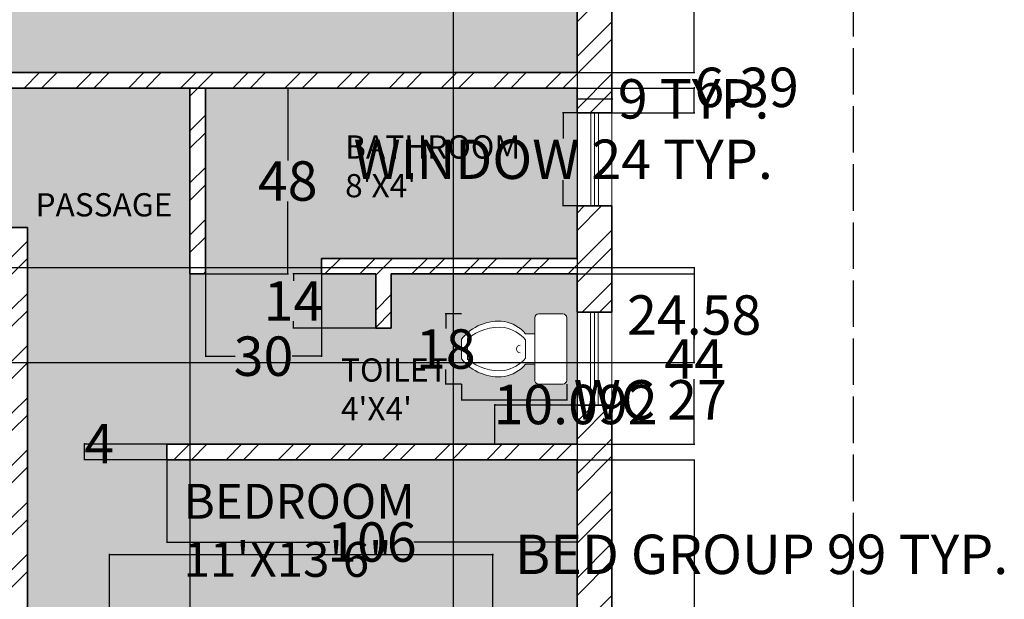
# Model space of a CAD drawing. Units: inches. Extents: x 1410 to 1959, y 5441 to 5968.
# Tile 4 of 5: x 1705 to 1959, y 5615 to 5765. Entities that reach past the tile are written whole.
import ezdxf

# ---------------------------------------------------------------- set-up
doc = ezdxf.new("R2010")
doc.units = ezdxf.units.IN
doc.linetypes.add('ACAD_ISO02W100', pattern=[15, 12, -3])
doc.layers.get('Defpoints').update_dxf_attribs({"linetype": 'ACAD_ISO02W100'})
for name, color, linetype, lineweight in [('A-ANNO-DIMS', 2, 'Continuous', 18), ('A-AREA-IDEN', 7, 'Continuous', 18), ('A-FLOR-FIXT', 9, 'Continuous', 18), ('A-WALL', 7, 'Continuous', 35), ('A-WALL-PATT', 8, 'Continuous', 13), ('WINDOW', 160, 'Continuous', 13)]:
    doc.layers.add(name, color=color, linetype=linetype, lineweight=lineweight)
doc.layers.add('A-FLOR-PATT', color=9, linetype='Continuous', lineweight=9, true_color=0xafd9aa)
doc.styles.get("Standard").update_dxf_attribs({"font": 'arial.ttf'})
doc.dimstyles.get("Standard").update_dxf_attribs({"dimtxt": 10.18, "dimasz": 0.18, "dimexe": 0.18, "dimexo": 0.0625, "dimgap": 0.09, "dimtad": 0, "dimtih": 1, "dimtoh": 1, "dimdec": 0, "dimzin": 0, "dimdsep": 46, "dimlunit": 3, "dimtxsty": 'Standard', "dimcen": 0.09, "dimadec": 0, "dimazin": 0, "dimtfac": 1, "dimtdec": 0, "dimtofl": 0, "dimtmove": 0, "dimatfit": 3, "dimfxl": 1, "dimtolj": 1, "dimtzin": 0, "dimarcsym": 0})

# ---------------------------------------------------------------- blocks, each defined once
blk = doc.blocks.new('A$C2AC94788')
for p, q in [((0, 0.505), (0, 0.665)), ((0.025, 0.69), (0.435, 0.69)), ((0.46, 0.665), (0.46, 0.505)), ((0.435, 0.48), (0.025, 0.48)), ((0.13, 0.48), (0.13, 0.42)), ((0.33, 0.42), (0.33, 0.48)), ((0.17, 0.42), (0.29, 0.42)), ((0.1641, 0.0392), (0.2959, 0.0392)), ((0.2291, 0.0392), (0.23, 0.0392)), ((0.2309, 0.0392), (0.23, 0.0392)), ((0.165, 0), (0.295, 0))]:
    blk.add_line(p, q)
for centre, radius, start, end in [((0.025, 0.665), 0.025, 90, 180), ((0.435, 0.665), 0.025, 0, 90), ((0.025, 0.505), 0.025, 180, 270), ((0.435, 0.505), 0.025, 270, 0), ((0.2874, 0.2356), 0.2425, 130.48854, 169.44501), ((0.3274, 0.2356), 0.2425, 130.48854, 169.44501), ((0.1326, 0.2356), 0.2425, 10.55499, 49.51146), ((0.1726, 0.2356), 0.2425, 10.55499, 49.51146), ((0.23, 0.385), 0.025, 180, 0), ((0.3601, 0.2448), 0.313, 173.53688, 231.44828), ((0.4001, 0.2448), 0.313, 173.53688, 221.06038), ((0.0999, 0.2448), 0.313, 308.55172, 6.46312), ((0.0599, 0.2448), 0.313, 318.93962, 6.46312)]:
    blk.add_arc(centre, radius, start, end)
blk = doc.blocks.new('WIN-24IN')
for p, q in [((3.5, 24), (3.5, 0)), ((4.5, 24), (4.5, 0)), ((5.5, 24), (5.5, 0))]:
    blk.add_line(p, q)
blk.add_lwpolyline([(0, 0), (9, 0), (9, 24), (0, 24)], close=True)
blk = doc.blocks.new('*D12')
at = {"layer": 'A-ANNO-DIMS', "color": 0, "lineweight": -2, "transparency": 16777216}
for p, q in [((1849.06, 5740.98), (1845.34, 5740.98)), ((1845.52, 5740.8), (1845.52, 5734.33)), ((1845.52, 5717.16), (1845.52, 5723.62)), ((1849.06, 5716.98), (1845.34, 5716.98))]:
    blk.add_line(p, q, dxfattribs=at)
at = {"layer": 'A-ANNO-DIMS', "color": 0, "transparency": 16777216}
for points in [[(1845.49, 5740.8), (1845.55, 5740.8), (1845.52, 5740.98)], [(1845.49, 5717.16), (1845.55, 5717.16), (1845.52, 5716.98)]]:
    blk.add_solid(points, dxfattribs=at)
at = {"layer": 'Defpoints', "color": 0, "transparency": 16777216}
for p in [(1845.52, 5740.98), (1849.12, 5740.98), (1849.12, 5716.98)]:
    blk.add_point(p, dxfattribs=at)
at = {"layer": 'A-ANNO-DIMS', "color": 0, "transparency": 16777216, "insert": (1845.52, 5728.98), "char_height": 10.18, "attachment_point": 5}
blk.add_mtext('\\A1;WINDOW 24 TYP.', dxfattribs=at)
blk = doc.blocks.new('*D13')
at = {"layer": 'A-ANNO-DIMS', "color": 0, "lineweight": -2, "transparency": 16777216}
for p, q in [((1849.12, 5741.04), (1849.12, 5744.76)), ((1849.3, 5744.58), (1857.94, 5744.58)), ((1858.12, 5741.04), (1858.12, 5744.76)), ((1858.12, 5744.58), (1858.3, 5744.58))]:
    blk.add_line(p, q, dxfattribs=at)
at = {"layer": 'A-ANNO-DIMS', "color": 0, "transparency": 16777216}
for points in [[(1849.3, 5744.61), (1849.3, 5744.55), (1849.12, 5744.58)], [(1857.94, 5744.61), (1857.94, 5744.55), (1858.12, 5744.58)]]:
    blk.add_solid(points, dxfattribs=at)
at = {"layer": 'Defpoints', "color": 0, "transparency": 16777216}
for p in [(1858.12, 5744.58), (1849.12, 5740.98), (1858.12, 5740.98)]:
    blk.add_point(p, dxfattribs=at)
at = {"layer": 'A-ANNO-DIMS', "color": 0, "transparency": 16777216, "insert": (1879.21, 5744.58), "char_height": 10.18, "attachment_point": 5}
blk.add_mtext('\\A1;9 TYP.', dxfattribs=at)
blk = doc.blocks.new('*D14')
at = {"layer": 'A-ANNO-DIMS', "color": 0, "lineweight": -2, "transparency": 16777216}
for p, q in [((1728.31, 5612.14), (1728.31, 5627.11)), ((1728.49, 5626.93), (1827.13, 5626.93)), ((1827.31, 5612.14), (1827.31, 5627.11)), ((1827.31, 5626.93), (1827.49, 5626.93))]:
    blk.add_line(p, q, dxfattribs=at)
at = {"layer": 'A-ANNO-DIMS', "color": 0, "transparency": 16777216}
for points in [[(1728.49, 5626.96), (1728.49, 5626.9), (1728.31, 5626.93)], [(1827.13, 5626.96), (1827.13, 5626.9), (1827.31, 5626.93)]]:
    blk.add_solid(points, dxfattribs=at)
at = {"layer": 'Defpoints', "color": 0, "transparency": 16777216}
for p in [(1827.31, 5626.93), (1728.31, 5612.08), (1827.31, 5612.08)]:
    blk.add_point(p, dxfattribs=at)
at = {"layer": 'A-ANNO-DIMS', "color": 0, "transparency": 16777216, "insert": (1896.77, 5626.93), "char_height": 10.18, "attachment_point": 5}
blk.add_mtext('\\A1;BED GROUP 99 TYP.', dxfattribs=at)
blk = doc.blocks.new('*D22')
at = {"layer": 'A-ANNO-DIMS', "color": 0, "lineweight": -2, "transparency": 16777216}
for p, q in [((1819.26, 5670.85), (1819.26, 5666.66)), ((1846.43, 5670.85), (1846.43, 5666.66)), ((1819.44, 5666.84), (1846.25, 5666.84)), ((1846.43, 5666.84), (1846.61, 5666.84))]:
    blk.add_line(p, q, dxfattribs=at)
at = {"layer": 'A-ANNO-DIMS', "color": 0, "transparency": 16777216}
for points in [[(1819.44, 5666.87), (1819.44, 5666.81), (1819.26, 5666.84)], [(1846.25, 5666.87), (1846.25, 5666.81), (1846.43, 5666.84)]]:
    blk.add_solid(points, dxfattribs=at)
at = {"layer": 'Defpoints', "color": 0, "transparency": 16777216}
for p in [(1819.26, 5670.92), (1846.43, 5670.92), (1846.43, 5666.84)]:
    blk.add_point(p, dxfattribs=at)
at = {"layer": 'A-ANNO-DIMS', "color": 0, "transparency": 16777216, "insert": (1868.02, 5666.84), "char_height": 10.18, "attachment_point": 5}
blk.add_mtext('\\A1;WC 27', dxfattribs=at)
blk = doc.blocks.new('*D23')
at = {"layer": 'A-ANNO-DIMS', "color": 0, "lineweight": -2, "transparency": 16777216}
for p, q in [((1819.2, 5689.03), (1815.01, 5689.03)), ((1815.19, 5688.85), (1815.19, 5685.26)), ((1815.19, 5671.1), (1815.19, 5674.68)), ((1819.2, 5670.92), (1815.01, 5670.92))]:
    blk.add_line(p, q, dxfattribs=at)
at = {"layer": 'A-ANNO-DIMS', "color": 0, "transparency": 16777216}
for points in [[(1815.16, 5688.85), (1815.22, 5688.85), (1815.19, 5689.03)], [(1815.16, 5671.1), (1815.22, 5671.1), (1815.19, 5670.92)]]:
    blk.add_solid(points, dxfattribs=at)
at = {"layer": 'Defpoints', "color": 0, "transparency": 16777216}
for p in [(1819.26, 5689.03), (1815.19, 5670.92), (1819.26, 5670.92)]:
    blk.add_point(p, dxfattribs=at)
at = {"layer": 'A-ANNO-DIMS', "color": 0, "transparency": 16777216, "insert": (1815.19, 5679.97), "char_height": 10.18, "attachment_point": 5}
blk.add_mtext('\\A1;18', dxfattribs=at)
blk = doc.blocks.new('*D28')
at = {"layer": 'A-ANNO-DIMS', "color": 0, "lineweight": -2, "transparency": 16777216}
for p, q in [((1817.1, 5913.3), (1817.1, 5478.87)), ((1849.09, 5913.3), (1849.09, 5478.87)), ((1817.28, 5479.05), (1848.91, 5479.05)), ((1849.09, 5479.05), (1849.27, 5479.05))]:
    blk.add_line(p, q, dxfattribs=at)
at = {"layer": 'A-ANNO-DIMS', "color": 0, "transparency": 16777216}
for points in [[(1817.28, 5479.08), (1817.28, 5479.02), (1817.1, 5479.05)], [(1848.91, 5479.08), (1848.91, 5479.02), (1849.09, 5479.05)]]:
    blk.add_solid(points, dxfattribs=at)
at = {"layer": 'Defpoints', "color": 0, "transparency": 16777216}
for p in [(1817.1, 5913.37), (1849.09, 5913.37), (1849.09, 5479.05)]:
    blk.add_point(p, dxfattribs=at)
at = {"layer": 'A-ANNO-DIMS', "color": 0, "transparency": 16777216, "insert": (1866.55, 5479.05), "char_height": 10.18, "attachment_point": 5}
blk.add_mtext('\\A1;31.99', dxfattribs=at)
blk = doc.blocks.new('*D32')
at = {"layer": 'A-ANNO-DIMS', "color": 0, "lineweight": -2, "transparency": 16777216}
for p, q in [((1849.03, 5665.46), (1827.66, 5665.46)), ((1827.84, 5665.46), (1827.84, 5665.64)), ((1827.84, 5665.64), (1828.02, 5665.64)), ((1827.84, 5655.55), (1827.84, 5665.28)), ((1849.03, 5655.37), (1827.66, 5655.37))]:
    blk.add_line(p, q, dxfattribs=at)
at = {"layer": 'A-ANNO-DIMS', "color": 0, "transparency": 16777216}
for points in [[(1827.81, 5665.28), (1827.87, 5665.28), (1827.84, 5665.46)], [(1827.81, 5655.55), (1827.87, 5655.55), (1827.84, 5655.37)]]:
    blk.add_solid(points, dxfattribs=at)
at = {"layer": 'Defpoints', "color": 0, "transparency": 16777216}
for p in [(1827.84, 5665.46), (1849.09, 5665.46), (1849.09, 5655.37)]:
    blk.add_point(p, dxfattribs=at)
at = {"layer": 'A-ANNO-DIMS', "color": 0, "transparency": 16777216, "insert": (1848.71, 5665.64), "char_height": 10.18, "attachment_point": 5}
blk.add_mtext('\\A1;10.092', dxfattribs=at)
blk = doc.blocks.new('*D33')
at = {"layer": 'A-ANNO-DIMS', "color": 0, "lineweight": -2, "transparency": 16777216}
for p, q in [((1849.16, 5747.37), (1879.55, 5747.37)), ((1879.37, 5747.37), (1879.37, 5747.55)), ((1879.37, 5747.55), (1879.55, 5747.55)), ((1879.37, 5741.16), (1879.37, 5747.19)), ((1849.19, 5740.98), (1879.55, 5740.98))]:
    blk.add_line(p, q, dxfattribs=at)
at = {"layer": 'A-ANNO-DIMS', "color": 0, "transparency": 16777216}
for points in [[(1879.34, 5747.19), (1879.4, 5747.19), (1879.37, 5747.37)], [(1879.34, 5741.16), (1879.4, 5741.16), (1879.37, 5740.98)]]:
    blk.add_solid(points, dxfattribs=at)
at = {"layer": 'Defpoints', "color": 0, "transparency": 16777216}
for p in [(1849.09, 5747.37), (1879.37, 5747.37), (1849.12, 5740.98)]:
    blk.add_point(p, dxfattribs=at)
at = {"layer": 'A-ANNO-DIMS', "color": 0, "transparency": 16777216, "insert": (1892.9, 5747.55), "char_height": 10.18, "attachment_point": 5}
blk.add_mtext('\\A1;6.39', dxfattribs=at)
blk = doc.blocks.new('*D41')
at = {"layer": 'A-ANNO-DIMS', "color": 0, "lineweight": -2, "transparency": 16777216}
for p, q in [((1849.16, 5651.37), (1879.55, 5651.37)), ((1879.37, 5651.19), (1879.37, 5598.65)), ((1879.37, 5535.55), (1879.37, 5588.08)), ((1849.16, 5535.37), (1879.55, 5535.37))]:
    blk.add_line(p, q, dxfattribs=at)
at = {"layer": 'A-ANNO-DIMS', "color": 0, "transparency": 16777216}
for points in [[(1879.34, 5651.19), (1879.4, 5651.19), (1879.37, 5651.37)], [(1879.34, 5535.55), (1879.4, 5535.55), (1879.37, 5535.37)]]:
    blk.add_solid(points, dxfattribs=at)
at = {"layer": 'Defpoints', "color": 0, "transparency": 16777216}
for p in [(1849.09, 5651.37), (1879.37, 5651.37), (1849.09, 5535.37)]:
    blk.add_point(p, dxfattribs=at)
at = {"layer": 'A-ANNO-DIMS', "color": 0, "transparency": 16777216, "insert": (1879.37, 5593.37), "char_height": 10.18, "attachment_point": 5}
blk.add_mtext('\\A1;116', dxfattribs=at)
blk = doc.blocks.new('*D43')
at = {"layer": 'A-ANNO-DIMS', "color": 0, "lineweight": -2, "transparency": 16777216}
for p, q in [((1849.16, 5913.37), (1879.55, 5913.37)), ((1879.37, 5913.19), (1879.37, 5837.65)), ((1879.37, 5751.55), (1879.37, 5827.08)), ((1849.16, 5751.37), (1879.55, 5751.37))]:
    blk.add_line(p, q, dxfattribs=at)
at = {"layer": 'A-ANNO-DIMS', "color": 0, "transparency": 16777216}
for points in [[(1879.34, 5913.19), (1879.4, 5913.19), (1879.37, 5913.37)], [(1879.34, 5751.55), (1879.4, 5751.55), (1879.37, 5751.37)]]:
    blk.add_solid(points, dxfattribs=at)
at = {"layer": 'Defpoints', "color": 0, "transparency": 16777216}
for p in [(1849.09, 5913.37), (1879.37, 5913.37), (1849.09, 5751.37)]:
    blk.add_point(p, dxfattribs=at)
at = {"layer": 'A-ANNO-DIMS', "color": 0, "transparency": 16777216, "insert": (1879.37, 5832.37), "char_height": 10.18, "attachment_point": 5}
blk.add_mtext('\\A1;162', dxfattribs=at)
blk = doc.blocks.new('*D44')
at = {"layer": 'A-ANNO-DIMS', "color": 0, "lineweight": -2, "transparency": 16777216}
for p, q in [((1753.09, 5699.3), (1753.09, 5677.94)), ((1783.09, 5699.3), (1783.09, 5677.94)), ((1753.27, 5678.12), (1760.73, 5678.12)), ((1782.91, 5678.12), (1775.45, 5678.12))]:
    blk.add_line(p, q, dxfattribs=at)
at = {"layer": 'A-ANNO-DIMS', "color": 0, "transparency": 16777216}
for points in [[(1753.27, 5678.15), (1753.27, 5678.09), (1753.09, 5678.12)], [(1782.91, 5678.15), (1782.91, 5678.09), (1783.09, 5678.12)]]:
    blk.add_solid(points, dxfattribs=at)
at = {"layer": 'Defpoints', "color": 0, "transparency": 16777216}
for p in [(1753.09, 5699.37), (1783.09, 5699.37), (1753.09, 5678.12)]:
    blk.add_point(p, dxfattribs=at)
at = {"layer": 'A-ANNO-DIMS', "color": 0, "transparency": 16777216, "insert": (1768.09, 5678.12), "char_height": 10.18, "attachment_point": 5}
blk.add_mtext('\\A1;30', dxfattribs=at)
blk = doc.blocks.new('*D45')
at = {"layer": 'A-ANNO-DIMS', "color": 0, "lineweight": -2, "transparency": 16777216}
for p, q in [((1797.03, 5699.37), (1775.66, 5699.37)), ((1775.84, 5699.19), (1775.84, 5697.57)), ((1775.84, 5685.55), (1775.84, 5687.17)), ((1797.03, 5685.37), (1775.66, 5685.37))]:
    blk.add_line(p, q, dxfattribs=at)
at = {"layer": 'A-ANNO-DIMS', "color": 0, "transparency": 16777216}
for points in [[(1775.81, 5699.19), (1775.87, 5699.19), (1775.84, 5699.37)], [(1775.81, 5685.55), (1775.87, 5685.55), (1775.84, 5685.37)]]:
    blk.add_solid(points, dxfattribs=at)
at = {"layer": 'Defpoints', "color": 0, "transparency": 16777216}
for p in [(1775.84, 5699.37), (1797.09, 5699.37), (1797.09, 5685.37)]:
    blk.add_point(p, dxfattribs=at)
at = {"layer": 'A-ANNO-DIMS', "color": 0, "transparency": 16777216, "insert": (1775.84, 5692.37), "char_height": 10.18, "attachment_point": 5}
blk.add_mtext('\\A1;14', dxfattribs=at)
blk = doc.blocks.new('*D46')
at = {"layer": 'A-ANNO-DIMS', "color": 0, "lineweight": -2, "transparency": 16777216}
for p, q in [((1707.09, 5711.3), (1707.09, 5478.87)), ((1749.09, 5699.3), (1749.09, 5478.87)), ((1707.27, 5479.05), (1720.56, 5479.05)), ((1748.91, 5479.05), (1735.63, 5479.05))]:
    blk.add_line(p, q, dxfattribs=at)
at = {"layer": 'A-ANNO-DIMS', "color": 0, "transparency": 16777216}
for points in [[(1707.27, 5479.08), (1707.27, 5479.02), (1707.09, 5479.05)], [(1748.91, 5479.08), (1748.91, 5479.02), (1749.09, 5479.05)]]:
    blk.add_solid(points, dxfattribs=at)
at = {"layer": 'Defpoints', "color": 0, "transparency": 16777216}
for p in [(1707.09, 5711.37), (1749.09, 5699.37), (1749.09, 5479.05)]:
    blk.add_point(p, dxfattribs=at)
at = {"layer": 'A-ANNO-DIMS', "color": 0, "transparency": 16777216, "insert": (1728.09, 5479.05), "char_height": 10.18, "attachment_point": 5}
blk.add_mtext('\\A1;42', dxfattribs=at)
blk = doc.blocks.new('*D47')
at = {"layer": 'A-ANNO-DIMS', "color": 0, "lineweight": -2, "transparency": 16777216}
for p, q in [((1707.03, 5747.37), (1685.66, 5747.37)), ((1685.84, 5747.19), (1685.84, 5734.66)), ((1685.84, 5711.55), (1685.84, 5724.07)), ((1707.03, 5711.37), (1685.66, 5711.37))]:
    blk.add_line(p, q, dxfattribs=at)
at = {"layer": 'A-ANNO-DIMS', "color": 0, "transparency": 16777216}
for points in [[(1685.81, 5747.19), (1685.87, 5747.19), (1685.84, 5747.37)], [(1685.81, 5711.55), (1685.87, 5711.55), (1685.84, 5711.37)]]:
    blk.add_solid(points, dxfattribs=at)
at = {"layer": 'Defpoints', "color": 0, "transparency": 16777216}
for p in [(1685.84, 5747.37), (1707.09, 5747.37), (1707.09, 5711.37)]:
    blk.add_point(p, dxfattribs=at)
at = {"layer": 'A-ANNO-DIMS', "color": 0, "transparency": 16777216, "insert": (1685.84, 5729.37), "char_height": 10.18, "attachment_point": 5}
blk.add_mtext('\\A1;36', dxfattribs=at)
blk = doc.blocks.new('*D48')
at = {"layer": 'A-ANNO-DIMS', "color": 0, "lineweight": -2, "transparency": 16777216}
for p, q in [((1743.09, 5651.3), (1743.09, 5629.94)), ((1849.09, 5651.3), (1849.09, 5629.94)), ((1743.27, 5630.12), (1785.24, 5630.12)), ((1848.91, 5630.12), (1806.95, 5630.12))]:
    blk.add_line(p, q, dxfattribs=at)
at = {"layer": 'A-ANNO-DIMS', "color": 0, "transparency": 16777216}
for points in [[(1743.27, 5630.15), (1743.27, 5630.09), (1743.09, 5630.12)], [(1848.91, 5630.15), (1848.91, 5630.09), (1849.09, 5630.12)]]:
    blk.add_solid(points, dxfattribs=at)
at = {"layer": 'Defpoints', "color": 0, "transparency": 16777216}
for p in [(1743.09, 5651.37), (1849.09, 5651.37), (1743.09, 5630.12)]:
    blk.add_point(p, dxfattribs=at)
at = {"layer": 'A-ANNO-DIMS', "color": 0, "transparency": 16777216, "insert": (1796.09, 5630.12), "char_height": 10.18, "attachment_point": 5}
blk.add_mtext('\\A1;106', dxfattribs=at)
blk = doc.blocks.new('*D56')
at = {"layer": 'A-ANNO-DIMS', "color": 0, "lineweight": -2, "transparency": 16777216}
for p, q in [((1743.03, 5655.37), (1721.66, 5655.37)), ((1721.84, 5655.37), (1721.84, 5655.55)), ((1721.84, 5655.55), (1722.02, 5655.55)), ((1721.84, 5651.55), (1721.84, 5655.19)), ((1743.03, 5651.37), (1721.66, 5651.37))]:
    blk.add_line(p, q, dxfattribs=at)
at = {"layer": 'A-ANNO-DIMS', "color": 0, "transparency": 16777216}
for points in [[(1721.81, 5655.19), (1721.87, 5655.19), (1721.84, 5655.37)], [(1721.81, 5651.55), (1721.87, 5651.55), (1721.84, 5651.37)]]:
    blk.add_solid(points, dxfattribs=at)
at = {"layer": 'Defpoints', "color": 0, "transparency": 16777216}
for p in [(1721.84, 5655.37), (1743.09, 5655.37), (1743.09, 5651.37)]:
    blk.add_point(p, dxfattribs=at)
at = {"layer": 'A-ANNO-DIMS', "color": 0, "transparency": 16777216, "insert": (1725.63, 5655.55), "char_height": 10.18, "attachment_point": 5}
blk.add_mtext('\\A1;4', dxfattribs=at)
blk = doc.blocks.new('*D57')
at = {"layer": 'A-ANNO-DIMS', "color": 0, "lineweight": -2, "transparency": 16777216}
for p, q in [((1753.16, 5747.37), (1774.52, 5747.37)), ((1774.34, 5747.19), (1774.34, 5728.65)), ((1774.34, 5699.55), (1774.34, 5718.08)), ((1753.16, 5699.37), (1774.52, 5699.37))]:
    blk.add_line(p, q, dxfattribs=at)
at = {"layer": 'A-ANNO-DIMS', "color": 0, "transparency": 16777216}
for points in [[(1774.31, 5747.19), (1774.37, 5747.19), (1774.34, 5747.37)], [(1774.31, 5699.55), (1774.37, 5699.55), (1774.34, 5699.37)]]:
    blk.add_solid(points, dxfattribs=at)
at = {"layer": 'Defpoints', "color": 0, "transparency": 16777216}
for p in [(1753.09, 5747.37), (1753.09, 5699.37), (1774.34, 5699.37)]:
    blk.add_point(p, dxfattribs=at)
at = {"layer": 'A-ANNO-DIMS', "color": 0, "transparency": 16777216, "insert": (1774.34, 5723.37), "char_height": 10.18, "attachment_point": 5}
blk.add_mtext('\\A1;48', dxfattribs=at)
blk = doc.blocks.new('*D58')
at = {"layer": 'A-ANNO-DIMS', "color": 0, "lineweight": -2, "transparency": 16777216}
for p, q in [((1849.156726, 5699.36591), (1879.553029, 5699.36591)), ((1879.373029, 5699.18591), (1879.373029, 5682.54591)), ((1879.373029, 5655.54591), (1879.373029, 5672.18591)), ((1849.156726, 5655.36591), (1879.553029, 5655.36591))]:
    blk.add_line(p, q, dxfattribs=at)
at = {"layer": 'A-ANNO-DIMS', "color": 0, "transparency": 16777216}
for points in [[(1879.343029, 5699.18591), (1879.403029, 5699.18591), (1879.373029, 5699.36591)], [(1879.343029, 5655.54591), (1879.403029, 5655.54591), (1879.373029, 5655.36591)]]:
    blk.add_solid(points, dxfattribs=at)
at = {"layer": 'Defpoints', "color": 0, "transparency": 16777216}
for p in [(1849.094226, 5699.36591), (1849.094226, 5655.36591), (1879.373029, 5655.36591)]:
    blk.add_point(p, dxfattribs=at)
at = {"layer": 'A-ANNO-DIMS', "color": 0, "transparency": 16777216, "insert": (1879.373029, 5677.36591), "char_height": 10.18, "attachment_point": 5}
blk.add_mtext('\\A1;44', dxfattribs=at)
blk = doc.blocks.new('*D59')
at = {"layer": 'A-ANNO-DIMS', "color": 0, "lineweight": -2, "transparency": 16777216}
for p, q in [((1559.15, 5701.04), (1879.55, 5701.04)), ((1879.37, 5700.86), (1879.37, 5694.04)), ((1879.37, 5676.64), (1879.37, 5683.46)), ((1559.15, 5676.46), (1879.55, 5676.46))]:
    blk.add_line(p, q, dxfattribs=at)
at = {"layer": 'A-ANNO-DIMS', "color": 0, "transparency": 16777216}
for points in [[(1879.34, 5700.86), (1879.4, 5700.86), (1879.37, 5701.04)], [(1879.34, 5676.64), (1879.4, 5676.64), (1879.37, 5676.46)]]:
    blk.add_solid(points, dxfattribs=at)
at = {"layer": 'Defpoints', "color": 0, "transparency": 16777216}
for p in [(1559.09, 5701.04), (1559.09, 5676.46), (1879.37, 5676.46)]:
    blk.add_point(p, dxfattribs=at)
at = {"layer": 'A-ANNO-DIMS', "color": 0, "transparency": 16777216, "insert": (1879.37, 5688.75), "char_height": 10.18, "attachment_point": 5}
blk.add_mtext('\\A1;24.58', dxfattribs=at)

msp = doc.modelspace()

# ---------------------------------------------------------------- hatches: boundary and pattern name
at = {"layer": 'A-FLOR-PATT', "transparency": 33554534}
h = msp.add_hatch(color=256, dxfattribs=at)
h.dxf.hatch_style = 1
h.paths.add_polyline_path([(1849.0942, 5913.3659), (1817.1029, 5913.3659), (1769.1029, 5913.3659), (1769.1029, 5913.3659), (1707.0942, 5913.3659), (1707.0942, 5787.3659), (1703.0942, 5787.3659), (1703.0942, 5799.3659), (1631.0942, 5799.3659), (1631.0942, 5787.3659), (1627.0942, 5787.3659), (1627.0942, 5889.3659), (1519.0989, 5889.3659), (1519.0989, 5816.4745), (1495.0981, 5816.4745), (1495.0981, 5809.856), (1495.0942, 5751.3659), (1631.0942, 5751.3659), (1631.0942, 5747.3659), (1495.0942, 5747.3659), (1495.0942, 5702.5811), (1495.0984, 5654.5768), (1495.0942, 5603.3659), (1667.0942, 5603.3659), (1667.0942, 5594.3659), (1650.778, 5594.3659), (1650.778, 5558.3659), (1703.0942, 5558.3659), (1703.0942, 5594.3659), (1703.0942, 5711.3659), (1707.0942, 5711.3659), (1707.0942, 5535.3659), (1754.5413, 5535.3659), (1802.541, 5535.3658), (1802.5413, 5535.3658), (1802.5413, 5535.3659), (1849.0942, 5535.3659), (1849.0942, 5651.3659), (1743.0942, 5651.3659), (1743.0942, 5655.3659), (1849.0942, 5655.3659), (1849.0942, 5665.4579), (1849.0942, 5689.4579), (1849.0942, 5699.3659), (1801.0942, 5699.3659), (1801.0942, 5685.3659), (1797.0942, 5685.3659), (1797.0942, 5699.3659), (1783.0942, 5699.3659), (1783.0942, 5703.3659), (1849.0942, 5703.3659), (1849.0942, 5716.9764), (1849.123, 5716.9764), (1849.123, 5740.9654), (1849.0942, 5740.9654), (1849.0942, 5747.3659), (1753.0942, 5747.3659), (1753.0942, 5699.3659), (1749.0942, 5699.3659), (1749.0942, 5747.3659), (1707.0942, 5747.3659), (1691.0942, 5747.3659), (1691.0942, 5751.3659), (1707.0942, 5751.3659), (1849.0942, 5751.3659)])
h.paths.add_polyline_path([(1533.4842, 5711.1518), (1533.4842, 5637.9201), (1534.7464, 5637.9201), (1534.7464, 5640.1099, -0.41421356), (1536.9363, 5642.2998), (1558.8347, 5642.2998, -0.41421356), (1561.0246, 5640.1099), (1561.0246, 5637.9201), (1563.2144, 5637.9201, -0.41421356), (1565.4042, 5635.7302), (1565.4042, 5609.4519, -0.41421356), (1563.2144, 5607.2621), (1532.5566, 5607.2621, -0.41421356), (1530.3668, 5609.4519), (1530.3668, 5635.4862), (1529.1045, 5635.4862), (1529.1045, 5633.2964, -0.41421356), (1526.9147, 5631.1065), (1500.6363, 5631.1065, -0.41421356), (1498.4465, 5633.2964), (1498.4465, 5715.5315, -0.41421356), (1500.6363, 5717.7213), (1526.9147, 5717.7213, -0.41421356), (1529.1045, 5715.5315), (1529.1045, 5713.3417), (1531.2944, 5713.3417, -0.41421356)], flags=16)
h.paths.add_polyline_path([(1771.0631, 5793.9619), (1771.0631, 5835.0118), (1771.0631, 5856.9619, -0.41421356), (1771.9631, 5857.8619), (1842.1181, 5857.8619, -0.41421356), (1843.0181, 5856.9619), (1843.0181, 5857.8619), (1846.6631, 5857.8619), (1846.6631, 5793.0619), (1843.0181, 5793.0619), (1828.4381, 5793.0619), (1771.9631, 5793.0619, -0.41421356)], flags=16)
h.paths.add_polyline_path([(1771.0631, 5805.9671, 0.25346465), (1781.0166, 5803.0153, 0.25379956), (1783.9781, 5793.0522)], flags=16)
h.paths.add_polyline_path([(1746.3058, 5612.0795), (1768.2559, 5612.0795), (1809.3058, 5612.0795, -0.41421356), (1810.2058, 5611.1795), (1810.2058, 5554.7045), (1810.2058, 5540.1245), (1810.2058, 5536.4795), (1745.4058, 5536.4795), (1745.4058, 5540.1245), (1746.3058, 5540.1245, -0.41421356), (1745.4058, 5541.0245), (1745.4058, 5611.1795, -0.41421356)], flags=16)
h.paths.add_polyline_path([(1819.5646, 5793.1537), (1819.5646, 5793.8054, 0.05271893), (1808.0815, 5849.0458, 0.29223153), (1819.5646, 5857.6981), (1828.4381, 5857.6981), (1828.4381, 5857.0464), (1828.4381, 5847.601, -0.06332793), (1838.1593, 5837.9401, -0.38046479), (1838.3062, 5835.5217, -0.02593615), (1834.5989, 5831.2824, -0.02509022), (1838.1593, 5827.1584, -0.38046478), (1838.3062, 5824.74, -0.05941785), (1829.2061, 5815.646, -0.11763956), (1828.4381, 5815.2914), (1828.4381, 5793.1537)], flags=0)
h.paths.add_polyline_path([(1819.5646, 5793.1537), (1819.5646, 5822.5662, -0.01603557), (1817.3363, 5825.2436, -0.4295765), (1817.4052, 5827.8865, -0.01537126), (1819.5646, 5830.4335), (1819.5646, 5833.3479, -0.01603557), (1817.3363, 5836.0254, -0.48413611), (1817.6682, 5838.8652, 0.00079305), (1817.0318, 5838.199, 0.26524804), (1817.0526, 5836.3926, 0.02736634), (1820.9176, 5831.8795, 0.02734261), (1817.0221, 5827.3996, 0.26229506), (1817.0526, 5825.6108, 0.06555279), (1827.0712, 5815.5721), (1827.0712, 5793.1537)], flags=0)
h.paths.add_polyline_path([(1830.4631, 5775.9619), (1830.4631, 5792.1619), (1846.6631, 5792.1619), (1846.6631, 5775.9619)], flags=16)
h.paths.add_polyline_path([(1831.3631, 5776.8619), (1831.3631, 5791.2619), (1845.7631, 5791.2619), (1845.7631, 5776.8619)], flags=0)
h.paths.add_polyline_path([(1836.6983, 5784.1006, -1), (1843.9547, 5784.1006, -1)], flags=0)
h.paths.add_polyline_path([(1819.2615, 5682.5311, -0.25820517), (1830.2865, 5687.0962, -0.1716359), (1835.799, 5683.9093), (1838.1615, 5683.9093), (1838.1615, 5688.0436, -0.41421356), (1839.1458, 5689.028), (1845.4458, 5689.028, -0.41421356), (1846.4302, 5688.0436), (1846.4302, 5671.8999, -0.41421356), (1845.4458, 5670.9155), (1839.1458, 5670.9155, -0.41421356), (1838.1615, 5671.8999), (1838.1615, 5676.0343), (1835.799, 5676.0343, -0.1716359), (1830.2865, 5672.8474, -0.25820517), (1819.2615, 5677.4124)], flags=16)
h.paths.add_polyline_path([(1820.8043, 5682.5681, -0.21038447), (1830.2865, 5685.5212, -0.1716359), (1835.799, 5682.3343), (1835.799, 5677.6093, -0.1716359), (1830.2865, 5674.4224, -0.21038447), (1820.8043, 5677.3755)], flags=0)
h.paths.add_polyline_path([(1842.0614, 5784.0231), (1841.8811, 5784.0231, -0.54460611), (1839.6163, 5782.7155), (1839.5262, 5782.5594, 0.54796211)], flags=0)
h.paths.add_polyline_path([(1840.3713, 5784.1781), (1840.3265, 5784.2556), (1840.2818, 5784.1781)], flags=0)
h.paths.add_polyline_path([(1830.4631, 5858.7619), (1830.4631, 5874.9619), (1846.6631, 5874.9619), (1846.6631, 5858.7619)], flags=16)
h.paths.add_polyline_path([(1831.3631, 5859.6619), (1831.3631, 5874.0619), (1845.7631, 5874.0619), (1845.7631, 5859.6619)], flags=0)
h.paths.add_polyline_path([(1755.6206, 5556.6903, -0.00089292), (1756.3396, 5557.4382), (1745.5695, 5557.4382), (1745.5695, 5554.7045), (1746.2212, 5554.7045), (1755.5673, 5554.7045, -0.38881883)], flags=0)
h.paths.add_polyline_path([(1810.114, 5563.578), (1810.114, 5554.7045), (1809.4622, 5554.7045), (1787.9762, 5554.7045, -0.11778508), (1787.6251, 5553.9338, -0.05941785), (1778.5249, 5544.8398, -0.37985907), (1776.1092, 5544.9833, -0.02509022), (1771.9852, 5548.5437, 0.03343123), (1776.8399, 5553.9365, 0.30845915), (1776.98, 5555.985, 0.04782679), (1769.9197, 5563.578), (1772.8341, 5563.578, -0.01537126), (1775.3811, 5565.7373, -0.4295765), (1778.024, 5565.8063, -0.01603557), (1780.7015, 5563.578)], flags=0)
h.paths.add_polyline_path([(1728.3058, 5552.6795), (1744.5058, 5552.6795), (1744.5058, 5536.4795), (1728.3058, 5536.4795)], flags=16)
h.paths.add_polyline_path([(1810.2058, 5599.1742, 0.25346465), (1800.2523, 5602.126, 0.25379956), (1797.2908, 5612.0892)], flags=16)
h.paths.add_polyline_path([(1843.9547, 5866.8231, -1), (1836.6983, 5866.8231, -1)], flags=0)
h.paths.add_polyline_path([(1729.2058, 5551.7795), (1743.6058, 5551.7795), (1743.6058, 5537.3795), (1729.2058, 5537.3795)], flags=0)
h.paths.add_polyline_path([(1839.4821, 5865.5155), (1840.237, 5866.8231), (1839.4821, 5868.1307, 0.25464572), (1838.77, 5866.8231, 0.25464572)], flags=0)
h.paths.add_polyline_path([(1842.0614, 5866.7456), (1840.3713, 5866.7456), (1839.5262, 5865.2819, 0.54796211)], flags=0)
h.paths.add_polyline_path([(1732.8163, 5542.8161, -1), (1740.0727, 5542.8161, -1)], flags=0)
h.paths.add_polyline_path([(1737.8296, 5543.5262), (1736.522, 5542.7713), (1736.522, 5541.2615, 0.39969799), (1738.001, 5542.8161, 0.11900365)], flags=0)
h.paths.add_polyline_path([(1738.1811, 5542.8161, -1), (1734.7079, 5542.8161, -1)], flags=0)
h.paths.add_polyline_path([(1736.4445, 5542.9056), (1736.367, 5542.9503), (1736.367, 5542.8608)], flags=0)
h.paths.add_polyline_path([(1811.1058, 5552.6795), (1827.3058, 5552.6795), (1827.3058, 5536.4795), (1811.1058, 5536.4795)], flags=16)
h.paths.add_polyline_path([(1812.0058, 5551.7795), (1826.4058, 5551.7795), (1826.4058, 5537.3795), (1812.0058, 5537.3795)], flags=0)
h.paths.add_polyline_path([(1815.5388, 5542.8161, -1), (1822.7952, 5542.8161, -1)], flags=0)
h.paths.add_polyline_path([(1820.5521, 5543.5262), (1819.2445, 5542.7713), (1819.2445, 5541.2615, 0.39969799), (1820.7235, 5542.8161, 0.11900365)], flags=0)
h.paths.add_polyline_path([(1820.9036, 5542.8161, -1), (1817.4304, 5542.8161, -1)], flags=0)
h.paths.add_polyline_path([(1819.167, 5542.9056), (1819.0895, 5542.9503), (1819.0895, 5542.8608)], flags=0)
h.paths.add_polyline_path([(1707.0264, 5710.8395), (1750.0905, 5710.8395), (1750.0905, 5723.2037), (1707.0264, 5723.2037)], flags=25)
h.paths.add_polyline_path([(1786.4108, 5658.162), (1818.7518, 5658.162), (1818.7518, 5680.5262), (1786.4108, 5680.5262)], flags=24)
h.paths.add_polyline_path([(1787.0609, 5715.7465), (1838.4906, 5715.7465), (1838.4906, 5738.1353), (1787.0609, 5738.1353)], flags=24)
h.paths.add_polyline_path([(1743.8116, 5616.0244), (1813.7243, 5616.0244), (1813.7243, 5649.6076), (1743.8116, 5649.6076)], flags=24)
h.paths.add_polyline_path([(1719.2569, 5867.7974), (1789.1696, 5867.7974), (1789.1696, 5901.3806), (1719.2569, 5901.3806)], flags=24)
h.paths.add_polyline_path([(1562.3198, 5677.907), (1619.4324, 5677.907), (1619.4324, 5711.4902), (1562.3198, 5711.4902)], flags=24)
h.paths.add_polyline_path([(1544.1706, 5816.5955), (1604.3036, 5816.5955), (1604.3036, 5850.1787), (1544.1706, 5850.1787)], flags=24)
at = {"layer": 'A-WALL-PATT'}
h = msp.add_hatch(dxfattribs=at)
h.set_pattern_fill('ANSI32', color=256)
h.paths.add_polyline_path([(1526.9987, 5922.3659), (1486.0942, 5922.3659), (1486.0942, 5857.8561), (1495.0942, 5857.8561), (1495.0942, 5913.3659), (1526.9987, 5913.3659)])
h.paths.add_polyline_path([(1769.1029, 5922.3659), (1574.9987, 5922.3659), (1574.9987, 5913.3659), (1574.9993, 5913.3659), (1627.0942, 5913.3659), (1627.0942, 5787.3659), (1631.0942, 5787.3659), (1631.0942, 5913.3659), (1703.0942, 5913.3659), (1703.0942, 5787.3659), (1707.0942, 5787.3659), (1707.0942, 5913.3659), (1769.1029, 5913.3659)])
h.paths.add_polyline_path([(1858.0942, 5922.3659), (1817.1029, 5922.3659), (1817.1029, 5913.3659), (1849.0942, 5913.3659), (1849.0942, 5751.3659), (1707.0942, 5751.3659), (1691.0942, 5751.3659), (1691.0942, 5747.3659), (1707.0942, 5747.3659), (1849.0942, 5747.3659), (1849.0942, 5740.9764), (1858.0942, 5740.9764)])
h.paths.add_polyline_path([(1495.0942, 5809.8561), (1486.0981, 5809.8561), (1486.0981, 5809.856), (1486.0942, 5702.5811), (1495.0942, 5702.5811), (1495.0942, 5747.3659), (1631.0942, 5747.3659), (1631.0942, 5751.3659), (1495.0942, 5751.3659)])
h.paths.add_polyline_path([(1495.0942, 5654.5811), (1486.0984, 5654.5811), (1486.0984, 5654.5768), (1486.0942, 5594.3659), (1667.0942, 5594.3659), (1667.0942, 5603.3659), (1495.0942, 5603.3659)])
h.paths.add_polyline_path([(1858.0942, 5665.4579), (1849.0942, 5665.4579), (1849.0942, 5655.3659), (1743.0942, 5655.3659), (1743.0942, 5651.3659), (1849.0942, 5651.3659), (1849.0942, 5535.3659), (1802.5413, 5535.3659), (1802.5413, 5526.3659), (1858.0942, 5526.3659)])
h.paths.add_polyline_path([(1858.0942, 5716.9654), (1849.0942, 5716.9654), (1849.0942, 5703.3659), (1783.0942, 5703.3659), (1783.0942, 5699.3659), (1797.0942, 5699.3659), (1797.0942, 5685.3659), (1801.0942, 5685.3659), (1801.0942, 5699.3659), (1849.0942, 5699.3659), (1849.0942, 5689.4579), (1858.0942, 5689.4579)])
h.paths.add_polyline_path([(1753.0942, 5747.3659), (1749.0942, 5747.3659), (1749.0942, 5699.3659), (1753.0942, 5699.3659)])
h.paths.add_polyline_path([(1707.0942, 5711.3659), (1703.0942, 5711.3659), (1703.0942, 5594.3659), (1703.0942, 5526.3659), (1754.5413, 5526.3659), (1754.5413, 5535.3658), (1754.541, 5535.3658), (1707.0942, 5535.3659)])

# ---------------------------------------------------------------- linework, layer by layer
at = {"layer": 'A-WALL'}
for p, q in [((1858.0942, 5922.3659), (1858.0942, 5740.9654)), ((1849.0942, 5913.3659), (1849.0942, 5751.3659)), ((1691.0942, 5751.3659), (1707.0942, 5751.3659)), ((1707.0942, 5751.3659), (1849.0942, 5751.3659)), ((1691.0942, 5747.3659), (1707.0942, 5747.3659)), ((1707.0942, 5747.3659), (1849.0942, 5747.3659)), ((1749.0942, 5747.3659), (1749.0942, 5699.3659)), ((1753.0942, 5747.3659), (1753.0942, 5699.3659)), ((1849.0942, 5747.3659), (1849.0942, 5740.9654)), ((1849.0942, 5740.9654), (1858.0942, 5740.9654)), ((1849.0942, 5716.9654), (1858.0942, 5716.9654)), ((1849.0942, 5716.9654), (1849.0942, 5703.3659)), ((1858.0942, 5716.9654), (1858.0942, 5689.4579)), ((1703.0942, 5711.3659), (1707.0942, 5711.3659)), ((1707.0942, 5711.3659), (1707.0942, 5535.3659)), ((1849.0942, 5703.3659), (1783.0942, 5703.3659)), ((1783.0942, 5703.3659), (1783.0942, 5699.3659)), ((1753.0942, 5699.3659), (1749.0942, 5699.3659)), ((1797.0942, 5699.3659), (1783.0942, 5699.3659)), ((1797.0942, 5699.3659), (1797.0942, 5685.3659)), ((1849.0942, 5699.3659), (1801.0942, 5699.3659)), ((1801.0942, 5699.3659), (1801.0942, 5685.3659)), ((1849.0942, 5699.3659), (1849.0942, 5689.4579)), ((1849.0942, 5689.4579), (1858.0942, 5689.4579)), ((1801.0942, 5685.3659), (1797.0942, 5685.3659)), ((1849.0942, 5665.4579), (1858.0942, 5665.4579)), ((1849.0942, 5665.4579), (1849.0942, 5655.3659)), ((1858.0942, 5665.4579), (1858.0942, 5526.3659)), ((1849.0942, 5655.3659), (1743.0942, 5655.3659)), ((1743.0942, 5655.3659), (1743.0942, 5651.3659)), ((1849.0942, 5651.3659), (1743.0942, 5651.3659)), ((1849.0942, 5651.3659), (1849.0942, 5535.3659))]:
    msp.add_line(p, q, dxfattribs=at)
at = {"layer": 'Defpoints'}
msp.add_lwpolyline([(1409.7428, 5967.6887), (1920.4745, 5967.6887), (1920.4745, 5440.571), (1409.7428, 5440.571)], close=True, dxfattribs=at)

# ---------------------------------------------------------------- block references
at = {"layer": 'A-FLOR-FIXT', "xscale": 39.375, "yscale": 39.375, "zscale": 39.375, "rotation": 270}
msp.add_blockref('A$C2AC94788', (1819.2615, 5689.028), dxfattribs=at)
at = {"layer": 'WINDOW'}
for p in [(1849.123, 5716.9764), (1849.0942, 5665.4579)]:
    msp.add_blockref('WIN-24IN', p, dxfattribs=at)

# ---------------------------------------------------------------- texts
at = {"layer": 'A-AREA-IDEN', "attachment_point": 1}
for s, width, insert, char_height in [("BATHROOM\\P8'X4'", 131.314672, (1789.1748, 5735.1537), 6), ('PASSAGE', 131.314672, (1709.173, 5720.218), 6), ("TOILET\\P4'X4'", 131.314672, (1788.1072, 5677.5447), 6), ('BEDROOM\\P11\'X13\'6"', 124.909089, (1747.4307, 5645.1353), 9)]:
    msp.add_mtext_dynamic_manual_height_columns(s, width=width, gutter_width=12.5, heights=[0], dxfattribs=dict(at, insert=insert, char_height=char_height))

# ---------------------------------------------------------------- dimensions: what is measured, and where the dimension line sits
at = {"layer": 'A-ANNO-DIMS'}
for base, p1, p2, override, picture, middle in [((1849.0942, 5479.0498), (1817.1029, 5913.3659), (1849.0942, 5913.3659), {"dimdec": 2, "dimlfac": 1, "dimrnd": 0, "dimzin": 0, "dimdsep": 46, "dimlunit": 2}, '*D28', (1866.5473, 5479.0498)), ((1749.0942, 5479.0498), (1707.0942, 5711.3659), (1749.0942, 5699.3659), {"dimdec": 0, "dimlfac": 1, "dimrnd": 0, "dimzin": 0, "dimdsep": 46, "dimlunit": 2}, '*D46', (1728.0942, 5479.0498))]:
    dim = msp.add_linear_dim(base=base, p1=p1, p2=p2, dimstyle='Standard', override=override, dxfattribs=at)
    dim.commit()
    dim.dimension.update_dxf_attribs({"geometry": picture, "text_midpoint": middle})
for base, p1, p2, angle, override, picture, middle in [((1879.373, 5913.3659), (1849.0942, 5751.3659), (1849.0942, 5913.3659), 90, {"dimdec": 0, "dimlfac": 1, "dimrnd": 0, "dimzin": 0, "dimdsep": 46, "dimlunit": 2}, '*D43', (1879.373, 5832.3659)), ((1879.373, 5747.3659), (1849.123, 5740.9764), (1849.0942, 5747.3659), 90, {"dimdec": 2, "dimlfac": 1, "dimrnd": 0, "dimzin": 0, "dimdsep": 46, "dimlunit": 2}, '*D33', (1892.9027, 5747.5459)), ((1685.8442, 5747.3659), (1707.0942, 5711.3659), (1707.0942, 5747.3659), 90, {"dimdec": 0, "dimlfac": 1, "dimrnd": 0, "dimzin": 0, "dimdsep": 46, "dimlunit": 2}, '*D47', (1685.8442, 5729.3659)), ((1774.3442, 5699.3659), (1753.0942, 5747.3659), (1753.0942, 5699.3659), 270, {"dimdec": 0, "dimlfac": 1, "dimrnd": 0, "dimzin": 0, "dimdsep": 46, "dimlunit": 2}, '*D57', (1774.3442, 5723.3659)), ((1879.373, 5676.4614), (1559.091, 5701.0417), (1559.091, 5676.4614), 90, {"dimdec": 2, "dimlfac": 1, "dimrnd": 0, "dimzin": 0, "dimdsep": 46, "dimlunit": 2}, '*D59', (1879.373, 5688.7515)), ((1753.0942, 5678.1159), (1783.0942, 5699.3659), (1753.0942, 5699.3659), 180, {"dimdec": 0, "dimlfac": 1, "dimrnd": 0, "dimzin": 0, "dimdsep": 46, "dimlunit": 2}, '*D44', (1768.0942, 5678.1159)), ((1775.8442, 5699.3659), (1797.0942, 5685.3659), (1797.0942, 5699.3659), 90, {"dimdec": 0, "dimlfac": 1, "dimrnd": 0, "dimzin": 0, "dimdsep": 46, "dimlunit": 2}, '*D45', (1775.8442, 5692.3659)), ((1879.373, 5655.3659), (1849.0942, 5699.3659), (1849.0942, 5655.3659), 90, {"dimdec": 0, "dimlfac": 1, "dimrnd": 0, "dimzin": 0, "dimdsep": 46, "dimlunit": 2}, '*D58', (1879.373, 5677.3659)), ((1815.1861, 5670.9155), (1819.2615, 5689.028), (1819.2615, 5670.9155), 270, {"dimdec": 0, "dimlfac": 1, "dimrnd": 0, "dimzin": 0, "dimdsep": 46, "dimlunit": 2}, '*D23', (1815.1861, 5679.9718)), ((1827.8442, 5665.4579), (1849.0942, 5655.3659), (1849.0942, 5665.4579), 90, {"dimdec": 3, "dimlfac": 1, "dimrnd": 0, "dimzin": 0, "dimdsep": 46, "dimlunit": 2}, '*D32', (1848.7138, 5665.6379)), ((1721.8442, 5655.3659), (1743.0942, 5651.3659), (1743.0942, 5655.3659), 90, {"dimdec": 0, "dimlfac": 1, "dimrnd": 0, "dimzin": 0, "dimdsep": 46, "dimlunit": 2}, '*D56', (1725.6349, 5655.5459)), ((1743.0942, 5630.1159), (1849.0942, 5651.3659), (1743.0942, 5651.3659), 180, {"dimdec": 0, "dimlfac": 1, "dimrnd": 0, "dimzin": 0, "dimdsep": 46, "dimlunit": 2}, '*D48', (1796.0942, 5630.1159)), ((1879.373, 5651.3659), (1849.0942, 5535.3659), (1849.0942, 5651.3659), 90, {"dimdec": 0, "dimlfac": 1, "dimrnd": 0, "dimzin": 0, "dimdsep": 46, "dimlunit": 2}, '*D41', (1879.373, 5593.3659))]:
    dim = msp.add_linear_dim(base=base, p1=p1, p2=p2, angle=angle, dimstyle='Standard', override=override, dxfattribs=at)
    dim.commit()
    dim.dimension.update_dxf_attribs({"geometry": picture, "text_midpoint": middle})
for base, p1, p2, text, picture, middle in [((1858.123, 5744.5764), (1849.123, 5740.9764), (1858.123, 5740.9764), '<> TYP.', '*D13', (1879.2148, 5744.5764)), ((1846.4302, 5666.8402), (1819.2615, 5670.9155), (1846.4302, 5670.9155), 'WC <>', '*D22', (1868.022, 5666.8402)), ((1827.3058, 5626.9295), (1728.3058, 5612.0795), (1827.3058, 5612.0795), 'BED GROUP <> TYP.', '*D14', (1896.7734, 5626.9295))]:
    dim = msp.add_linear_dim(base=base, p1=p1, p2=p2, text=text, dimstyle='Standard', override={"dimdec": 0, "dimlfac": 1, "dimrnd": 0, "dimzin": 0, "dimdsep": 46, "dimlunit": 2}, dxfattribs=at)
    dim.commit()
    dim.dimension.update_dxf_attribs({"geometry": picture, "text_midpoint": middle})
dim = msp.add_linear_dim(base=(1845.523, 5740.9764), p1=(1849.123, 5716.9764), p2=(1849.123, 5740.9764), angle=90, text='WINDOW <> TYP.', dimstyle='Standard', override={"dimdec": 0, "dimlfac": 1, "dimrnd": 0, "dimzin": 0, "dimdsep": 46, "dimlunit": 2}, dxfattribs=at)
dim.commit()
dim.dimension.update_dxf_attribs({"geometry": '*D12', "text_midpoint": (1845.523, 5728.9764)})

doc.saveas('drawing.dxf')
